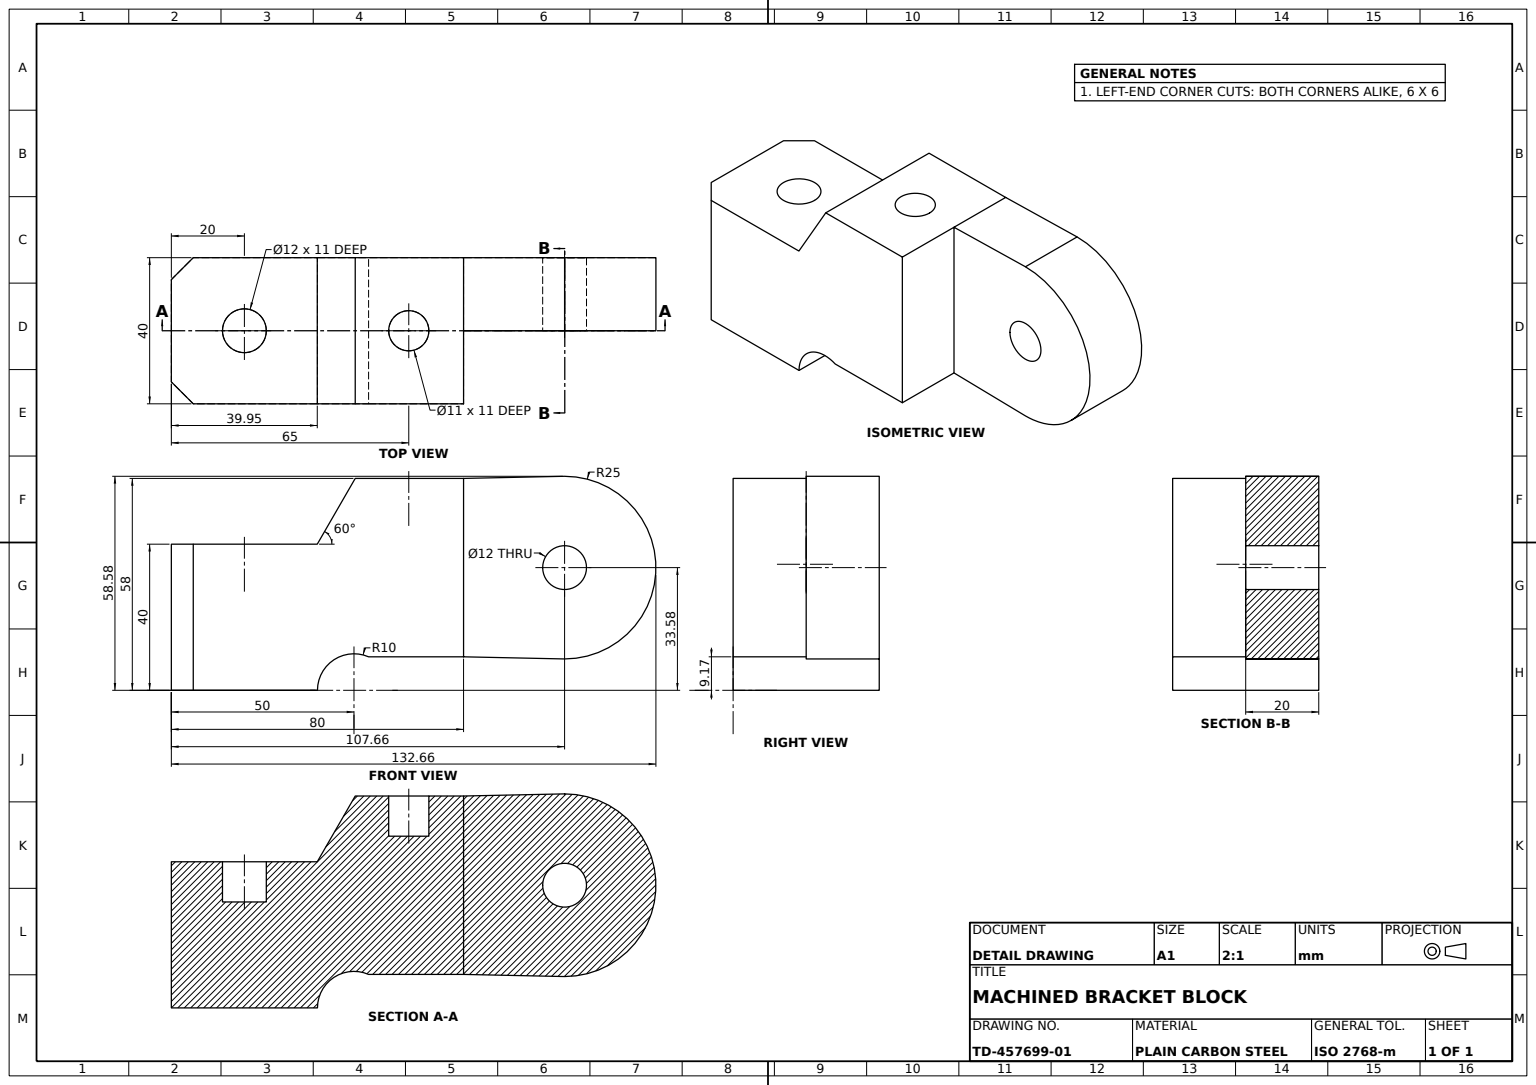
SolidWorks part; units mm, degrees
material "Plain Carbon Steel"
ref_plane "Front Plane" through (0, 0, 0) normal (0, 0, 1) x (1, 0, 0)
ref_plane "Top Plane" through (0, 0, 0) normal (0, 1, 0) x (1, 0, 0)
ref_plane "Right Plane" through (0, 0, 0) normal (1, 0, 0) x (0, 0, -1)
sketch "Housing Profile Sketch" plane through (0, 0, 0) normal (1, 0, 0) x (0, 0, -1)
  line L0 (0, 0) -> (40, 0)
  line L1 (54, 9.1652) -> (80, 9.1652)
  line L2 (80, 9.1652) -> (80, 58)
  line L3 (80, 58) -> (50.3414, 58)
  line L4 (50.3414, 58) -> (39.9491, 40)
  line L5 (39.9491, 40) -> (0, 40)
  line L6 (0, 40) -> (0, 0)
  line L7 (50.3414, 58) -> (6.2008, 58) construction
  arc A0 (40, 0) -> (54, 9.1652) centre (50, 0) cw
  dimension "D3" = 10
  dimension "D1" = 80
  dimension "D2" = 40
  dimension "D4" = 26
  dimension "D5" = 58
  dimension "D6" = 40
  dimension "D7" = 60
  dimension "D8" = 29.6586
extrude "Housing Body" add sketch "Housing Profile Sketch" along normal mid plane 40
sketch "Corner Cut A Sketch" plane through (0, 0, 0) normal (0, -1, 0) x (1, 0, 0)
  line L0 (0, 0) -> (0, -40) construction
  line L1 (20, -40) -> (-20, -40) construction
  line L2 (14, 0) -> (20, -6)
  line L3 (20, 0) -> (-20, 0) construction
  line L4 (20, 0) -> (20, -40) construction
  line L5 (20, -6) -> (20, 0)
  line L6 (20, 0) -> (14, 0)
  line L7 (-20, 0) -> (-14, 0)
  line L8 (-20, -6) -> (-20, 0)
  line L9 (-14, 0) -> (-20, -6)
  dimension "D1" = 6
  dimension "D2" = 6
extrude "Corner Cut A 6x6" cut sketch "Corner Cut A Sketch" against normal through all contours L2 L5 L6
sketch "Corner Cut B Sketch" plane through (0, 0, 0) normal (0, -1, 0) x (1, 0, 0)
  line L0 (-20, 0) -> (-20, -6)
  line L2 (-20, 0) -> (-20, -40) construction
  line L3 (-20, -6) -> (-14, 0)
  line L4 (14, 0) -> (-20, 0) construction
  line L5 (-14, 0) -> (-20, 0)
  dimension "D1" = 6
  dimension "D2" = 6
extrude "Corner Cut B 6x6" cut sketch "Corner Cut B Sketch" against normal through all contours L3 L5 L0
sketch "Step Hole Sketch" plane through (0, 40, 0) normal (0, 1, 0) x (1, 0, 0)
  line L0 (14, 0) -> (-14, 0) construction
  line L1 (-20, 39.9491) -> (-20, 6) construction
  circle A0 centre (0, 20) radius 6
  dimension "D2" = 12
  dimension "D1" = 20
  dimension "D3" = 20
extrude "Step Hole Cut" cut sketch "Step Hole Sketch" against normal blind 11
sketch "Second Step Cut Sketch" plane through (0, 58, 0) normal (0, 1, 0) x (1, 0, 0)
  line L0 (0, 20) -> (-20, 20) construction
  line L1 (-20, 39.9491) -> (-20, 6) construction
  circle A0 centre (0, 65) radius 5.5
  dimension "D2" = 11
  dimension "D1" = 45
extrude "Second Step Cut" cut sketch "Second Step Cut Sketch" against normal blind 11
sketch "Eye Lug Sketch" plane through (-20, 0, 0) normal (-1, 0, 0) x (0, 0, 1)
  line L0 (-107.6573, 58.5826) -> (-80, 58)
  line L1 (-80, 58) -> (-80, 9.1652)
  line L2 (-80, 9.1652) -> (-107.6573, 8.5826)
  line L4 (-6, 40) -> (-6, 0) construction
  arc A0 (-107.6573, 58.5826) -> (-107.6573, 8.5826) centre (-107.6573, 33.5826) ccw
  dimension "D1" = 50
  dimension "D2" = 101.6573
extrude "Eye Lug" add sketch "Eye Lug Sketch" against normal blind 20 contours A0 L2 L1 L0
sketch "Eye Bore Sketch" plane through (0, 0, 0) normal (1, 0, 0) x (0, 0, -1)
  circle A0 centre (107.6573, 33.5826) radius 6
  dimension "D1" = 12
extrude "Eye Bore Ø12" cut sketch "Eye Bore Sketch" against normal through all
